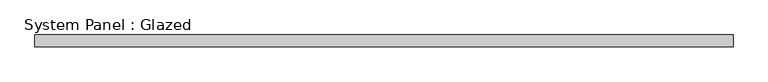
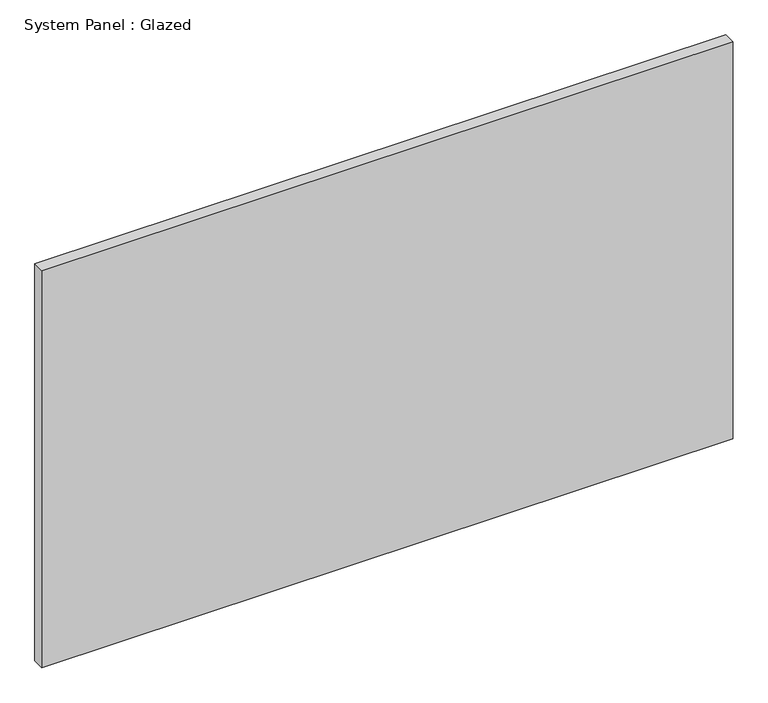
"""IFC4 building model written with IfcOpenShell, lengths in millimetres: plate geometry, System Panel : Glazed."""

from ifc_helpers import new_model, si_unit, origin, origin_with_axes, place, context, project, spatial, polyline, outline, extrude, source, transform, mapped, element, save


def system_panel_glazed_524f965d(model_context):
    return source(origin(), model_context, "Body", "SweptSolid", [
        extrude(outline(polyline([(753.0205134, 19.05), (-753.0205134, 19.05), (-753.0205134, 44.45), (753.0205134, 44.45), (753.0205134, 19.05)])), origin_with_axes(), (0.0, 0.0, 1.0), 914.4),
    ])


if __name__ == "__main__":
    model = new_model("IFC4")
    model_context = context("Model", 3, world=origin())
    ifc_project = project(units=[si_unit("LENGTHUNIT", "METRE", prefix="MILLI")], contexts=[model_context])
    site = spatial("IfcSite", under=ifc_project)
    building = spatial("IfcBuilding", under=site)
    placement = place(None, origin())
    system_panel_glazed_shape = system_panel_glazed_524f965d(model_context)
    element("IfcPlate", 1, ObjectType="System Panel : Glazed", at=placement, inside=building, context=model_context, shape_type="MappedRepresentation", body=[
        mapped(system_panel_glazed_shape, transform((0.0, 0.0, 0.0), x_axis=(1.0, 0.0, 0.0), y_axis=(0.0, 1.0, 0.0), z_axis=(0.0, 0.0, 1.0))),
    ])
    save(model, "model.ifc")

# Revit data of these elements
# Type "System Panel : Glazed"
#   Construction Type Id = "GSP4R"
#   Analytic Construction = "1/8 in Pilkington single glazing"
#   Visual Light Transmittance = 0.9
#   Solar Heat Gain Coefficient = 0.86
#   Heat Transfer Coefficient (U) = 6.7069 W/(m²·K)
# Element 1 (IfcPlate, "System Panel : Glazed")
#   Materials on its faces: "Glass"
# Materials
#   "Glass": class "Glass", colour RGB 0 128 192, transparency 0.75, Description = "Soda Lime Glass", Cost = 0
